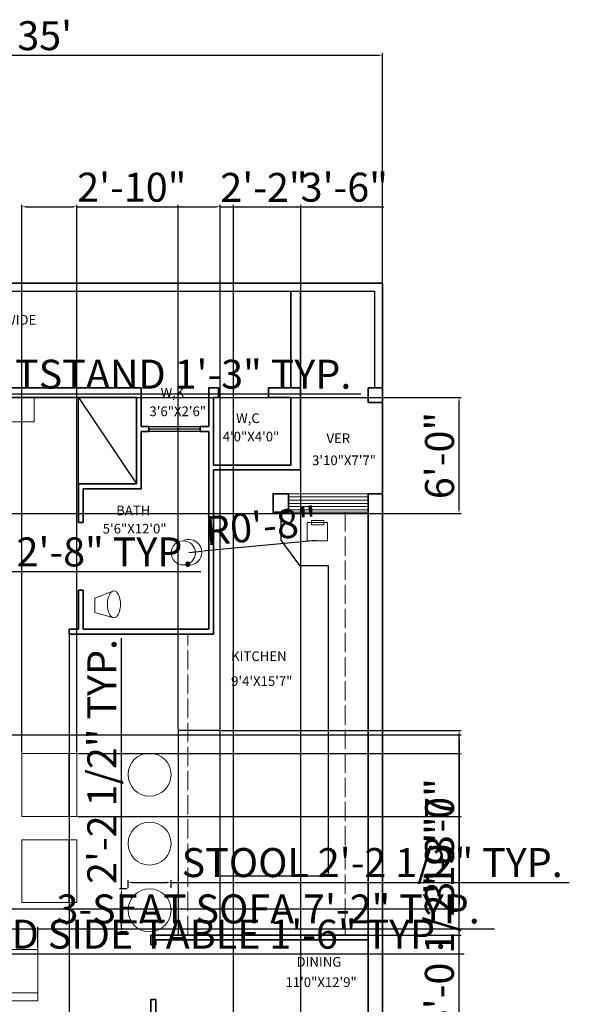
# Model space of a CAD drawing. Units: inches. Extents: x 2484 to 3244, y 1684 to 2692.
# Tile 3 of 3: x 2821 to 3162, y 2081 to 2692. Entities that reach past the tile are written whole.
import ezdxf

# ---------------------------------------------------------------- set-up
doc = ezdxf.new("R2010")
doc.units = ezdxf.units.IN
doc.linetypes.add('ACAD_ISO02W100', pattern=[15, 12, -3])
doc.layers.get('0').update_dxf_attribs({"color": 120})
for name, color, linetype, lineweight in [('A-ANNO-DIMS', 2, 'Continuous', 18), ('A-AREA-IDEN', 2, 'Continuous', 18), ('A-COLS', 120, 'Continuous', 35), ('A-FLOR-CASE', 120, 'Continuous', 25), ('A-FLOR-CASE-OVHD', 255, 'ACAD_ISO02W100', 18), ('A-FLOR-FIXT', 4, 'Continuous', 18), ('A-FURN', 40, 'Continuous', 18), ('A-GLAZ', 4, 'Continuous', 13), ('A-WALL', 120, 'Continuous', 35), ('A-WALL-OVHD', 255, 'ACAD_ISO02W100', 18), ('C-PROP', 120, 'Continuous', 35), ('C-SITE', 120, 'Continuous', 25)]:
    doc.layers.add(name, color=color, linetype=linetype, lineweight=lineweight)
doc.styles.get("Standard").update_dxf_attribs({"font": 'arial.ttf'})
doc.dimstyles.new('ISO-25', dxfattribs={"dimtxt": 18, "dimasz": 2.5, "dimexe": 1.25, "dimexo": 0.625, "dimtad": 1, "dimdec": 0, "dimlunit": 3, "dimtxsty": 'Standard', "dimcen": 2.5, "dimadec": 0, "dimazin": 0, "dimtfac": 1, "dimtdec": 0, "dimtmove": 0, "dimatfit": 3, "dimfxl": 1, "dimarcsym": 0})

# ---------------------------------------------------------------- blocks, each defined once
blk = doc.blocks.new('*D1')
at = {"layer": 'A-ANNO-DIMS', "color": 0, "lineweight": -2, "transparency": 16777216}
for p, q in [((2626.09, 2529.34), (2626.09, 2671.64)), ((2628.59, 2670.39), (3043.59, 2670.39)), ((3046.09, 2529.34), (3046.09, 2671.64))]:
    blk.add_line(p, q, dxfattribs=at)
at = {"layer": 'A-ANNO-DIMS', "color": 0, "transparency": 16777216}
for points in [[(2628.59, 2670.81), (2628.59, 2669.97), (2626.09, 2670.39)], [(3043.59, 2670.81), (3043.59, 2669.97), (3046.09, 2670.39)]]:
    blk.add_solid(points, dxfattribs=at)
at = {"layer": 'Defpoints', "color": 0, "transparency": 16777216}
for p in [(3046.09, 2670.39), (2626.09, 2528.71), (3046.09, 2528.71)]:
    blk.add_point(p, dxfattribs=at)
at = {"layer": 'A-ANNO-DIMS', "color": 0, "transparency": 16777216, "insert": (2836.09, 2680.21), "char_height": 18, "attachment_point": 5}
blk.add_mtext("35'", dxfattribs=at)
blk = doc.blocks.new('SOFA-3')
for p, q in [((0.07, 0), (0.07, 32)), ((0.07, 32), (86.07, 32)), ((29.07, 0), (29.07, 32)), ((58.07, 0), (58.07, 32)), ((86.07, 32), (86.07, 0)), ((0.07, 0), (0, 5)), ((0, 5), (86.07, 5)), ((0.07, 0), (0.07, 5)), ((86.07, 0), (0.07, 0))]:
    blk.add_line(p, q)
blk = doc.blocks.new('STOOL')
blk.add_circle((0, 0), 13.36)
blk = doc.blocks.new('NIGHTSTAND-15')
blk.add_lwpolyline([(15, 15), (0, 15), (0, 0), (15, 0)], close=True)
blk = doc.blocks.new('*D9')
at = {"layer": 'A-ANNO-DIMS', "color": 0, "lineweight": -2, "transparency": 16777216}
for p, q in [((2714.44, 2109.91), (2714.44, 2113.27)), ((2716.94, 2112.02), (2730.14, 2112.02)), ((2732.64, 2109.91), (2732.64, 2113.27)), ((2732.64, 2112.02), (3096.69, 2112.02))]:
    blk.add_line(p, q, dxfattribs=at)
at = {"layer": 'A-ANNO-DIMS', "color": 0, "transparency": 16777216}
for points in [[(2716.94, 2112.44), (2716.94, 2111.6), (2714.44, 2112.02)], [(2730.14, 2112.44), (2730.14, 2111.6), (2732.64, 2112.02)]]:
    blk.add_solid(points, dxfattribs=at)
at = {"layer": 'Defpoints', "color": 0, "transparency": 16777216}
for p in [(2732.64, 2112.02), (2714.44, 2109.29), (2732.64, 2109.29)]:
    blk.add_point(p, dxfattribs=at)
at = {"layer": 'A-ANNO-DIMS', "color": 0, "transparency": 16777216, "insert": (2915.92, 2121.96), "char_height": 18, "attachment_point": 5}
blk.add_mtext('ROUND SIDE TABLE 1\'-6" TYP.', dxfattribs=at)
blk = doc.blocks.new('*D11')
at = {"layer": 'A-ANNO-DIMS', "color": 0, "lineweight": -2, "transparency": 16777216}
for p, q in [((2887.88, 2153.12), (2887.88, 2157.76)), ((2890.38, 2156.51), (2912.09, 2156.51)), ((2914.59, 2153.12), (2914.59, 2157.76)), ((2914.59, 2156.51), (3162.14, 2156.51))]:
    blk.add_line(p, q, dxfattribs=at)
at = {"layer": 'A-ANNO-DIMS', "color": 0, "transparency": 16777216}
for points in [[(2890.38, 2156.92), (2890.38, 2156.09), (2887.88, 2156.51)], [(2912.09, 2156.92), (2912.09, 2156.09), (2914.59, 2156.51)]]:
    blk.add_solid(points, dxfattribs=at)
at = {"layer": 'Defpoints', "color": 0, "transparency": 16777216}
for p in [(2914.59, 2156.51), (2887.88, 2152.5), (2914.59, 2152.5)]:
    blk.add_point(p, dxfattribs=at)
at = {"layer": 'A-ANNO-DIMS', "color": 0, "transparency": 16777216, "insert": (3039.62, 2166.45), "char_height": 18, "attachment_point": 5}
blk.add_mtext('STOOL 2\'-2 1/2" TYP.', dxfattribs=at)
blk = doc.blocks.new('*D12')
at = {"layer": 'A-ANNO-DIMS', "color": 0, "lineweight": -2, "transparency": 16777216}
for p, q in [((2883.87, 2152.5), (2883.87, 2308.22)), ((2887.25, 2152.5), (2882.62, 2152.5)), ((2883.87, 2128.28), (2883.87, 2150)), ((2887.25, 2125.78), (2882.62, 2125.78))]:
    blk.add_line(p, q, dxfattribs=at)
at = {"layer": 'A-ANNO-DIMS', "color": 0, "transparency": 16777216}
for points in [[(2883.45, 2150), (2884.29, 2150), (2883.87, 2152.5)], [(2883.45, 2128.28), (2884.29, 2128.28), (2883.87, 2125.78)]]:
    blk.add_solid(points, dxfattribs=at)
at = {"layer": 'Defpoints', "color": 0, "transparency": 16777216}
for p in [(2883.87, 2152.5), (2887.88, 2152.5), (2887.88, 2125.78)]:
    blk.add_point(p, dxfattribs=at)
at = {"layer": 'A-ANNO-DIMS', "color": 0, "transparency": 16777216, "insert": (2873.94, 2231.61), "char_height": 18, "attachment_point": 5, "rotation": 90}
blk.add_mtext('2\'-2 1/2" TYP.', dxfattribs=at)
blk = doc.blocks.new('*D13')
at = {"layer": 'A-ANNO-DIMS', "color": 0, "lineweight": -2, "transparency": 16777216}
for p, q in [((2745.68, 2115.42), (2745.68, 2128.95)), ((2831.75, 2115.42), (2831.75, 2128.95)), ((2748.18, 2127.7), (2829.25, 2127.7)), ((2831.75, 2127.7), (3115.68, 2127.7))]:
    blk.add_line(p, q, dxfattribs=at)
at = {"layer": 'A-ANNO-DIMS', "color": 0, "transparency": 16777216}
for points in [[(2748.18, 2128.12), (2748.18, 2127.28), (2745.68, 2127.7)], [(2829.25, 2128.12), (2829.25, 2127.28), (2831.75, 2127.7)]]:
    blk.add_solid(points, dxfattribs=at)
at = {"layer": 'Defpoints', "color": 0, "transparency": 16777216}
for p in [(2831.75, 2127.7), (2745.68, 2114.79), (2831.75, 2114.79)]:
    blk.add_point(p, dxfattribs=at)
at = {"layer": 'A-ANNO-DIMS', "color": 0, "transparency": 16777216, "insert": (2974.96, 2137.65), "char_height": 18, "attachment_point": 5}
blk.add_mtext('3-SEAT SOFA 7\'-2" TYP.', dxfattribs=at)
blk = doc.blocks.new('*D17')
at = {"layer": 'A-ANNO-DIMS', "color": 0, "lineweight": -2, "transparency": 16777216}
for p, q in [((2702.65, 2345.36), (2702.65, 2350.79)), ((2705.15, 2349.54), (2732.15, 2349.54)), ((2734.65, 2345.36), (2734.65, 2350.79)), ((2734.65, 2349.54), (2933.13, 2349.54))]:
    blk.add_line(p, q, dxfattribs=at)
at = {"layer": 'A-ANNO-DIMS', "color": 0, "transparency": 16777216}
for points in [[(2705.15, 2349.96), (2705.15, 2349.12), (2702.65, 2349.54)], [(2732.15, 2349.96), (2732.15, 2349.12), (2734.65, 2349.54)]]:
    blk.add_solid(points, dxfattribs=at)
at = {"layer": 'Defpoints', "color": 0, "transparency": 16777216}
for p in [(2734.65, 2349.54), (2702.65, 2344.74), (2734.65, 2344.74)]:
    blk.add_point(p, dxfattribs=at)
at = {"layer": 'A-ANNO-DIMS', "color": 0, "transparency": 16777216, "insert": (2835.14, 2359.47), "char_height": 18, "attachment_point": 5}
blk.add_mtext('CHAIR 2\'-8" TYP.', dxfattribs=at)
blk = doc.blocks.new('*D19')
at = {"layer": 'A-ANNO-DIMS', "color": 0, "lineweight": -2, "transparency": 16777216}
for p, q in [((2734.51, 2458.34), (2734.51, 2461.21)), ((2737.01, 2459.96), (2747.01, 2459.96)), ((2749.51, 2458.34), (2749.51, 2461.21)), ((2749.51, 2459.96), (3032.54, 2459.96))]:
    blk.add_line(p, q, dxfattribs=at)
at = {"layer": 'A-ANNO-DIMS', "color": 0, "transparency": 16777216}
for points in [[(2737.01, 2460.38), (2737.01, 2459.55), (2734.51, 2459.96)], [(2747.01, 2460.38), (2747.01, 2459.55), (2749.51, 2459.96)]]:
    blk.add_solid(points, dxfattribs=at)
at = {"layer": 'Defpoints', "color": 0, "transparency": 16777216}
for p in [(2749.51, 2459.96), (2734.51, 2457.71), (2749.51, 2457.71)]:
    blk.add_point(p, dxfattribs=at)
at = {"layer": 'A-ANNO-DIMS', "color": 0, "transparency": 16777216, "insert": (2892.27, 2469.9), "char_height": 18, "attachment_point": 5}
blk.add_mtext('NIGHTSTAND 1\'-3" TYP.', dxfattribs=at)
blk = doc.blocks.new('*D22')
at = {"layer": 'A-ANNO-DIMS', "color": 0, "lineweight": -2, "transparency": 16777216}
for p, q in [((2815.13, 2457.71), (3094.89, 2457.71)), ((3093.64, 2388.21), (3093.64, 2455.21)), ((2815.13, 2385.71), (3094.89, 2385.71))]:
    blk.add_line(p, q, dxfattribs=at)
at = {"layer": 'A-ANNO-DIMS', "color": 0, "transparency": 16777216}
for points in [[(3093.22, 2455.21), (3094.05, 2455.21), (3093.64, 2457.71)], [(3093.22, 2388.21), (3094.05, 2388.21), (3093.64, 2385.71)]]:
    blk.add_solid(points, dxfattribs=at)
at = {"layer": 'Defpoints', "color": 0, "transparency": 16777216}
for p in [(2814.51, 2457.71), (3093.64, 2457.71), (2814.51, 2385.71)]:
    blk.add_point(p, dxfattribs=at)
at = {"layer": 'A-ANNO-DIMS', "color": 0, "transparency": 16777216, "insert": (3083.82, 2421.71), "char_height": 18, "attachment_point": 5, "rotation": 90}
blk.add_mtext('6\'-0"', dxfattribs=at)
blk = doc.blocks.new('*D23')
at = {"layer": 'A-ANNO-DIMS', "color": 0, "lineweight": -2, "transparency": 16777216}
for p, q in [((2953.42, 2064.92), (2953.42, 2577.51)), ((2955.92, 2576.26), (2992.74, 2576.26)), ((2995.24, 2064.92), (2995.24, 2577.51)), ((2995.24, 2576.26), (3046.83, 2576.26))]:
    blk.add_line(p, q, dxfattribs=at)
at = {"layer": 'A-ANNO-DIMS', "color": 0, "transparency": 16777216}
for points in [[(2955.92, 2576.68), (2955.92, 2575.85), (2953.42, 2576.26)], [(2992.74, 2576.68), (2992.74, 2575.85), (2995.24, 2576.26)]]:
    blk.add_solid(points, dxfattribs=at)
at = {"layer": 'Defpoints', "color": 0, "transparency": 16777216}
for p in [(2995.24, 2576.26), (2953.42, 2064.3), (2995.24, 2064.3)]:
    blk.add_point(p, dxfattribs=at)
at = {"layer": 'A-ANNO-DIMS', "color": 0, "transparency": 16777216, "insert": (3022.28, 2586.08), "char_height": 18, "attachment_point": 5}
blk.add_mtext('3\'-6"', dxfattribs=at)
blk = doc.blocks.new('*D24')
at = {"layer": 'A-ANNO-DIMS', "color": 0, "lineweight": -2, "transparency": 16777216}
for p, q in [((3093.64, 2064.3), (3093.64, 2157.84)), ((2995.86, 2064.3), (3094.89, 2064.3)), ((3093.64, 2006.27), (3093.64, 2061.8)), ((2995.86, 2003.77), (3094.89, 2003.77))]:
    blk.add_line(p, q, dxfattribs=at)
at = {"layer": 'A-ANNO-DIMS', "color": 0, "transparency": 16777216}
for points in [[(3093.22, 2061.8), (3094.05, 2061.8), (3093.64, 2064.3)], [(3093.22, 2006.27), (3094.05, 2006.27), (3093.64, 2003.77)]]:
    blk.add_solid(points, dxfattribs=at)
at = {"layer": 'Defpoints', "color": 0, "transparency": 16777216}
for p in [(2995.24, 2064.3), (3093.64, 2064.3), (2995.24, 2003.77)]:
    blk.add_point(p, dxfattribs=at)
at = {"layer": 'A-ANNO-DIMS', "color": 0, "transparency": 16777216, "insert": (3083.71, 2112.32), "char_height": 18, "attachment_point": 5, "rotation": 90}
blk.add_mtext('5\'-0 1/2"', dxfattribs=at)
blk = doc.blocks.new('*D31')
at = {"layer": 'A-ANNO-DIMS', "color": 0, "lineweight": -2, "transparency": 16777216}
for p, q in [((2705.68, 2248.09), (3094.89, 2248.09)), ((3093.64, 2245.59), (3093.64, 2142.59)), ((2705.68, 2140.09), (3094.89, 2140.09))]:
    blk.add_line(p, q, dxfattribs=at)
at = {"layer": 'A-ANNO-DIMS', "color": 0, "transparency": 16777216}
for points in [[(3093.22, 2245.59), (3094.05, 2245.59), (3093.64, 2248.09)], [(3093.22, 2142.59), (3094.05, 2142.59), (3093.64, 2140.09)]]:
    blk.add_solid(points, dxfattribs=at)
at = {"layer": 'Defpoints', "color": 0, "transparency": 16777216}
for p in [(2705.05, 2248.09), (2705.05, 2140.09), (3093.64, 2140.09)]:
    blk.add_point(p, dxfattribs=at)
at = {"layer": 'A-ANNO-DIMS', "color": 0, "transparency": 16777216, "insert": (3083.82, 2194.09), "char_height": 18, "attachment_point": 5, "rotation": 90}
blk.add_mtext('9\'-0"', dxfattribs=at)
blk = doc.blocks.new('*D33')
at = {"layer": 'A-ANNO-DIMS', "color": 0, "lineweight": -2, "transparency": 16777216}
for p, q in [((2821.96, 2237.17), (2821.96, 2577.51)), ((2824.46, 2576.26), (2853.53, 2576.26)), ((2856.03, 2237.17), (2856.03, 2577.51)), ((2856.03, 2576.26), (2921.92, 2576.26))]:
    blk.add_line(p, q, dxfattribs=at)
at = {"layer": 'A-ANNO-DIMS', "color": 0, "transparency": 16777216}
for points in [[(2824.46, 2576.68), (2824.46, 2575.85), (2821.96, 2576.26)], [(2853.53, 2576.68), (2853.53, 2575.85), (2856.03, 2576.26)]]:
    blk.add_solid(points, dxfattribs=at)
at = {"layer": 'Defpoints', "color": 0, "transparency": 16777216}
for p in [(2856.03, 2576.26), (2821.96, 2236.54), (2856.03, 2236.54)]:
    blk.add_point(p, dxfattribs=at)
at = {"layer": 'A-ANNO-DIMS', "color": 0, "transparency": 16777216, "insert": (2890.23, 2586.08), "char_height": 18, "attachment_point": 5}
blk.add_mtext('2\'-10"', dxfattribs=at)
blk = doc.blocks.new('*D34')
at = {"layer": 'A-ANNO-DIMS', "color": 0, "lineweight": -2, "transparency": 16777216}
for p, q in [((2856.66, 2236.54), (3094.89, 2236.54)), ((3093.64, 2234.04), (3093.64, 2199.97)), ((2856.66, 2197.47), (3094.89, 2197.47)), ((3093.64, 2197.47), (3093.64, 2145.88))]:
    blk.add_line(p, q, dxfattribs=at)
at = {"layer": 'A-ANNO-DIMS', "color": 0, "transparency": 16777216}
for points in [[(3093.22, 2234.04), (3094.05, 2234.04), (3093.64, 2236.54)], [(3093.22, 2199.97), (3094.05, 2199.97), (3093.64, 2197.47)]]:
    blk.add_solid(points, dxfattribs=at)
at = {"layer": 'Defpoints', "color": 0, "transparency": 16777216}
for p in [(2856.03, 2236.54), (2856.03, 2197.47), (3093.64, 2197.47)]:
    blk.add_point(p, dxfattribs=at)
at = {"layer": 'A-ANNO-DIMS', "color": 0, "transparency": 16777216, "insert": (3083.82, 2170.43), "char_height": 18, "attachment_point": 5, "rotation": 90}
blk.add_mtext('3\'-3"', dxfattribs=at)
blk = doc.blocks.new('*D37')
at = {"layer": 'A-ANNO-DIMS', "color": 0, "lineweight": -2, "transparency": 16777216}
for p, q in [((2799.42, 2313.09), (2799.42, 1699.91)), ((2851.28, 2313.09), (2851.28, 1699.91)), ((2801.92, 1701.16), (2848.78, 1701.16))]:
    blk.add_line(p, q, dxfattribs=at)
at = {"layer": 'A-ANNO-DIMS', "color": 0, "transparency": 16777216}
for points in [[(2801.92, 1701.58), (2801.92, 1700.75), (2799.42, 1701.16)], [(2848.78, 1701.58), (2848.78, 1700.75), (2851.28, 1701.16)]]:
    blk.add_solid(points, dxfattribs=at)
at = {"layer": 'Defpoints', "color": 0, "transparency": 16777216}
for p in [(2799.42, 2313.71), (2851.28, 2313.71), (2851.28, 1701.16)]:
    blk.add_point(p, dxfattribs=at)
at = {"layer": 'A-ANNO-DIMS', "color": 0, "transparency": 16777216, "insert": (2825.35, 1710.79), "char_height": 18, "attachment_point": 5}
blk.add_mtext('4\'-4"', dxfattribs=at)
blk = doc.blocks.new('*D39')
at = {"layer": 'A-ANNO-DIMS', "color": 0, "lineweight": -2, "transparency": 16777216}
for p, q in [((2919.09, 2251.56), (2919.09, 2577.51)), ((2921.59, 2576.26), (2942.66, 2576.26)), ((2945.16, 2251.56), (2945.16, 2577.51)), ((2945.16, 2576.26), (2997.07, 2576.26))]:
    blk.add_line(p, q, dxfattribs=at)
at = {"layer": 'A-ANNO-DIMS', "color": 0, "transparency": 16777216}
for points in [[(2921.59, 2576.68), (2921.59, 2575.85), (2919.09, 2576.26)], [(2942.66, 2576.68), (2942.66, 2575.85), (2945.16, 2576.26)]]:
    blk.add_solid(points, dxfattribs=at)
at = {"layer": 'Defpoints', "color": 0, "transparency": 16777216}
for p in [(2945.16, 2576.26), (2919.09, 2250.94), (2945.16, 2250.94)]:
    blk.add_point(p, dxfattribs=at)
at = {"layer": 'A-ANNO-DIMS', "color": 0, "transparency": 16777216, "insert": (2972.36, 2585.93), "char_height": 18, "attachment_point": 5}
blk.add_mtext('2\'-2"', dxfattribs=at)
blk = doc.blocks.new('*D40')
at = {"layer": 'A-ANNO-DIMS', "color": 0, "lineweight": -2, "transparency": 16777216}
for p, q in [((2945.79, 2250.94), (3094.89, 2250.94)), ((3093.64, 2126.21), (3093.64, 2248.44)), ((2945.79, 2123.71), (3094.89, 2123.71))]:
    blk.add_line(p, q, dxfattribs=at)
at = {"layer": 'A-ANNO-DIMS', "color": 0, "transparency": 16777216}
for points in [[(3093.22, 2248.44), (3094.05, 2248.44), (3093.64, 2250.94)], [(3093.22, 2126.21), (3094.05, 2126.21), (3093.64, 2123.71)]]:
    blk.add_solid(points, dxfattribs=at)
at = {"layer": 'Defpoints', "color": 0, "transparency": 16777216}
for p in [(2945.16, 2250.94), (3093.64, 2250.94), (2945.16, 2123.71)]:
    blk.add_point(p, dxfattribs=at)
at = {"layer": 'A-ANNO-DIMS', "color": 0, "transparency": 16777216, "insert": (3083.82, 2187.33), "char_height": 18, "attachment_point": 5, "rotation": 90}
blk.add_mtext('10\'-7"', dxfattribs=at)
blk = doc.blocks.new('*D41')
at = {"layer": 'A-ANNO-DIMS', "color": 0, "lineweight": -2, "transparency": 16777216}
for p, q in [((3004.71, 2368.85), (2936.18, 2362.5)), ((2925.73, 2361.54), (2933.69, 2362.27))]:
    blk.add_line(p, q, dxfattribs=at)
at = {"layer": 'A-ANNO-DIMS', "color": 0, "transparency": 16777216}
blk.add_solid([(2936.14, 2362.92), (2936.22, 2362.09), (2933.69, 2362.27)], dxfattribs=at)
at = {"layer": 'Defpoints', "color": 0, "transparency": 16777216}
for p in [(2925.73, 2361.54), (2933.69, 2362.27)]:
    blk.add_point(p, dxfattribs=at)
at = {"layer": 'A-ANNO-DIMS', "color": 0, "transparency": 16777216, "insert": (2970.79, 2375.57), "char_height": 18, "attachment_point": 5, "rotation": 5.28891}
blk.add_mtext('R0\'-8"', dxfattribs=at)

msp = doc.modelspace()

# ---------------------------------------------------------------- linework, layer by layer
at = {"layer": 'A-COLS'}
msp.add_lwpolyline([(2987.58, 2397.94), (2977.99, 2397.94), (2977.99, 2386.45), (2987.58, 2386.45)], close=True, dxfattribs=at)
at = {"layer": 'A-FLOR-CASE'}
for p, q in [((2857.09, 2404.08), (2857.09, 2457.71)), ((2857.09, 2457.71), (2893.09, 2404.08)), ((2982.78, 2386.45), (2982.78, 2369.09)), ((2982.78, 2369.09), (2994.39, 2353.45)), ((2994.39, 2353.45), (3012.33, 2353.45)), ((3012.33, 2353.45), (3012.33, 2160.37)), ((3012.33, 2160.37), (2945.16, 2160.37))]:
    msp.add_line(p, q, dxfattribs=at)
msp.add_lwpolyline([(2919.09, 2123.71), (2945.16, 2123.71), (2945.16, 2250.94), (2919.09, 2250.94)], close=True, dxfattribs=at)
at = {"layer": 'A-FLOR-CASE-OVHD'}
msp.add_line((3022.92, 2386.45), (3022.92, 2123.71), dxfattribs=at)
at = {"layer": 'A-FLOR-FIXT'}
for p, q in [((2879.13, 2337.66), (2867.27, 2333.03)), ((2867.27, 2333.03), (2867.27, 2324.07)), ((2867.27, 2324.07), (2879.13, 2320.89))]:
    msp.add_line(p, q, dxfattribs=at)
for points in [[(2999.24, 2380.02), (3011.92, 2380.02), (3011.92, 2368.62), (2999.24, 2368.62)], [(3001.93, 2381.25), (3009.65, 2381.25), (3009.65, 2378.63), (3001.93, 2378.63)]]:
    msp.add_lwpolyline(points, close=True, dxfattribs=at)
msp.add_circle((2922.22, 2361.21), 7.51, dxfattribs=at)
msp.add_arc((2925.73, 2361.54), 8, 254.60149, 115.98031, dxfattribs=at)
msp.add_ellipse((2879.13, 2329.28), major_axis=(0, -8.39), ratio=0.482758, dxfattribs=at)
at = {"layer": 'A-FURN'}
for p, q in [((2856.03, 2236.54), (2851.04, 2236.26)), ((2851.04, 2236.26), (2851.04, 2197.47)), ((2851.04, 2182.97), (2851.04, 2143.89))]:
    msp.add_line(p, q, dxfattribs=at)
for points in [[(2821.96, 2197.47), (2856.03, 2197.47), (2856.03, 2236.54), (2821.96, 2236.54)], [(2821.96, 2143.89), (2856.03, 2143.89), (2856.03, 2182.97), (2821.96, 2182.97)]]:
    msp.add_lwpolyline(points, close=True, dxfattribs=at)
at = {"layer": 'A-GLAZ'}
for p, q in [((2900.73, 2439.71), (2932.65, 2439.71)), ((2900.73, 2438.71), (2932.65, 2438.71)), ((2900.73, 2437.71), (2932.65, 2437.71)), ((2900.73, 2436.71), (2932.65, 2436.71)), ((2987.58, 2397.94), (3037.09, 2397.94)), ((2987.58, 2395.94), (3037.09, 2395.94)), ((2987.58, 2393.94), (3037.09, 2393.94)), ((2987.58, 2391.94), (3037.09, 2391.94)), ((2987.58, 2389.94), (3037.09, 2389.94)), ((2987.58, 2387.94), (3037.09, 2387.94)), ((2987.58, 2386.45), (3037.09, 2386.45))]:
    msp.add_line(p, q, dxfattribs=at)
at = {"layer": 'A-WALL'}
for p, q in [((2989.09, 2523.71), (2989.09, 2463.71)), ((2995.09, 2523.71), (2995.09, 2412.71)), ((2691.09, 2463.71), (2896.09, 2463.71)), ((2896.09, 2463.71), (2896.09, 2439.71)), ((2938.09, 2463.71), (2938.09, 2439.71)), ((2938.09, 2463.71), (2944.09, 2463.71)), ((2944.09, 2463.71), (2944.09, 2457.71)), ((2975.09, 2463.71), (2995.09, 2463.71)), ((2975.09, 2457.71), (2975.09, 2463.71)), ((3037.09, 2463.71), (3037.09, 2454.71)), ((3037.09, 2463.71), (3037.09, 2454.71)), ((3037.09, 2463.71), (3041.09, 2463.71)), ((3046.09, 2463.71), (3041.09, 2463.71)), ((3046.09, 2454.71), (3046.09, 2463.71)), ((2697.09, 2457.71), (2893.09, 2457.71)), ((2893.09, 2457.71), (2893.09, 2404.08)), ((2941.09, 2457.71), (2941.09, 2415.71)), ((2941.09, 2457.71), (2944.09, 2457.71)), ((2975.09, 2457.71), (2989.09, 2457.71)), ((2989.09, 2457.71), (2989.09, 2415.71)), ((3037.09, 2454.71), (3046.09, 2454.71)), ((2900.73, 2439.71), (2896.09, 2439.71)), ((2900.73, 2436.71), (2896.09, 2436.71)), ((2896.09, 2436.71), (2896.09, 2401.08)), ((2900.73, 2439.71), (2900.73, 2436.71)), ((2938.09, 2439.71), (2932.65, 2439.71)), ((2932.65, 2439.71), (2932.65, 2436.71)), ((2938.09, 2436.71), (2932.65, 2436.71)), ((2938.09, 2436.71), (2938.09, 2313.71)), ((2941.09, 2415.71), (2989.09, 2415.71)), ((2941.09, 2412.71), (2995.09, 2412.71)), ((2941.09, 2412.71), (2941.09, 2310.71)), ((2893.09, 2404.08), (2857.09, 2404.08)), ((2857.09, 2404.08), (2857.09, 2380.08)), ((2857.09, 2401.08), (2857.09, 2380.08)), ((2860.09, 2380.08), (2860.09, 2401.08)), ((2860.09, 2401.08), (2896.09, 2401.08)), ((2860.09, 2401.08), (2860.09, 2380.08)), ((3037.09, 2397.94), (3046.09, 2397.94)), ((3037.09, 2397.94), (3037.09, 1973.56)), ((2857.09, 2380.08), (2860.09, 2380.08)), ((2857.09, 2338.08), (2860.09, 2338.08)), ((2857.09, 2338.08), (2857.09, 2313.71)), ((2860.09, 2338.08), (2860.09, 2313.71)), ((2851.28, 2313.71), (2851.28, 2310.71)), ((2851.28, 2313.71), (2857.09, 2313.71)), ((2860.09, 2313.71), (2938.09, 2313.71)), ((2851.28, 2310.71), (2941.09, 2310.71)), ((2902.09, 2123.71), (3037.09, 2123.71)), ((2902.09, 2123.71), (2902.09, 2117.71)), ((2905.09, 2117.71), (2902.09, 2117.71)), ((2905.09, 2120.71), (3037.09, 2120.71)), ((2905.09, 2120.71), (2905.09, 2117.71)), ((2905.09, 2120.71), (2905.09, 2117.71)), ((2905.09, 2083.7), (2902.09, 2083.7)), ((2902.09, 2083.7), (2902.09, 2071.85)), ((2905.09, 2083.7), (2905.09, 2065.85))]:
    msp.add_line(p, q, dxfattribs=at)
at = {"layer": 'A-WALL-OVHD'}
for p, q in [((2919.09, 2310.71), (2919.09, 2123.71)), ((2925.09, 2123.71), (2925.09, 2310.71))]:
    msp.add_line(p, q, dxfattribs=at)
at = {"layer": 'C-PROP'}
msp.add_lwpolyline([(2626.09, 2528.71), (3046.09, 2528.71), (3046.09, 1748.71), (2626.09, 1748.71)], close=True, dxfattribs=at)
at = {"layer": 'C-SITE'}
for p, q in [((2631.09, 2523.71), (3041.09, 2523.71)), ((3041.09, 2523.71), (3041.09, 2463.71))]:
    msp.add_line(p, q, dxfattribs=at)

# ---------------------------------------------------------------- block references
at = {"layer": 'A-FURN'}
for name, p in [('NIGHTSTAND-15', (2814.51, 2442.71)), ('STOOL', (2901.24, 2223.44)), ('STOOL', (2901.24, 2180.6)), ('STOOL', (2901.24, 2139.14)), ('SOFA-3', (2745.68, 2082.79))]:
    msp.add_blockref(name, p, dxfattribs=at)

# ---------------------------------------------------------------- texts
at = {"layer": 'A-AREA-IDEN'}
for tag, p in [('5\'-4"WIDE', (2792.76, 2503.01)), ('W,K', (2908.14, 2457.7)), ('3\'6"X2\'6"', (2901.2, 2446.14)), ('W,C', (2955.05, 2441.88)), ('4\'0"X4\'0"', (2946.72, 2430.48)), ('VER', (3011.23, 2429.4)), ('3\'10"X7\'7"', (3002.28, 2415.71)), ('BATH', (2880.51, 2384.57)), ('5\'6"X12\'0"', (2872.13, 2373.25)), ('KITCHEN', (2951.94, 2294)), ('9\'4\'X15\'7"', (2951.94, 2278.53)), ('DINING', (2992.59, 2104.11)), ('11\'0"X12\'9"', (2985.76, 2091.49))]:
    msp.add_attdef(tag, p, '', height=6, dxfattribs=at)

# ---------------------------------------------------------------- dimensions: what is measured, and where the dimension line sits
at = {"layer": 'A-ANNO-DIMS'}
for base, p1, p2, override, picture, middle in [((3046.09, 2670.39), (2626.09, 2528.71), (3046.09, 2528.71), {"dimclrd": 0, "dimclre": 0, "dimclrt": 0}, '*D1', (2836.09, 2680.21)), ((2856.03, 2576.26), (2821.96, 2236.54), (2856.03, 2236.54), {"dimdec": 1, "dimlfac": 1, "dimrnd": 0, "dimzin": 1, "dimdsep": 46, "dimlunit": 4, "dimfrac": 2}, '*D33', (2890.23, 2586.08)), ((2945.16, 2576.26), (2919.09, 2250.94), (2945.16, 2250.94), {"dimdec": 1, "dimlfac": 1, "dimrnd": 0, "dimzin": 1, "dimdsep": 46, "dimlunit": 4, "dimfrac": 2}, '*D39', (2972.36, 2585.93)), ((2995.24, 2576.26), (2953.42, 2064.3), (2995.24, 2064.3), {"dimdec": 1, "dimlfac": 1, "dimrnd": 0, "dimzin": 1, "dimdsep": 46, "dimlunit": 4, "dimfrac": 2}, '*D23', (3022.28, 2586.08)), ((2851.28, 1701.16), (2799.42, 2313.71), (2851.28, 2313.71), {"dimdec": 1, "dimlfac": 1, "dimrnd": 0, "dimzin": 1, "dimdsep": 46, "dimlunit": 4, "dimfrac": 2}, '*D37', (2825.35, 1710.79))]:
    dim = msp.add_linear_dim(base=base, p1=p1, p2=p2, dimstyle='ISO-25', override=override, dxfattribs=at)
    dim.commit()
    dim.dimension.update_dxf_attribs({"geometry": picture, "text_midpoint": middle})
for base, p1, p2, text, picture, middle in [((2749.51, 2459.96), (2734.51, 2457.71), (2749.51, 2457.71), 'NIGHTSTAND <> TYP.', '*D19', (2892.27, 2469.9)), ((2734.65, 2349.54), (2702.65, 2344.74), (2734.65, 2344.74), 'CHAIR <> TYP.', '*D17', (2835.14, 2359.47)), ((2914.59, 2156.51), (2887.88, 2152.5), (2914.59, 2152.5), 'STOOL <> TYP.', '*D11', (3039.62, 2166.45)), ((2732.64, 2112.02), (2714.44, 2109.29), (2732.64, 2109.29), 'ROUND SIDE TABLE <> TYP.', '*D9', (2915.92, 2121.96)), ((2831.75, 2127.7), (2745.68, 2114.79), (2831.75, 2114.79), '3-SEAT SOFA <> TYP.', '*D13', (2974.96, 2137.65))]:
    dim = msp.add_linear_dim(base=base, p1=p1, p2=p2, text=text, dimstyle='ISO-25', override={"dimdec": 1, "dimlfac": 1, "dimrnd": 0, "dimzin": 1, "dimdsep": 46, "dimlunit": 4, "dimfrac": 2}, dxfattribs=at)
    dim.commit()
    dim.dimension.update_dxf_attribs({"geometry": picture, "text_midpoint": middle})
for base, p1, p2, picture, middle in [((3093.64, 2457.71), (2814.51, 2385.71), (2814.51, 2457.71), '*D22', (3083.82, 2421.71)), ((3093.64, 2140.09), (2705.05, 2248.09), (2705.05, 2140.09), '*D31', (3083.82, 2194.09)), ((3093.64, 2250.94), (2945.16, 2123.71), (2945.16, 2250.94), '*D40', (3083.82, 2187.33)), ((3093.64, 2197.47), (2856.03, 2236.54), (2856.03, 2197.47), '*D34', (3083.82, 2170.43)), ((3093.64, 2064.3), (2995.24, 2003.77), (2995.24, 2064.3), '*D24', (3083.71, 2112.32))]:
    dim = msp.add_linear_dim(base=base, p1=p1, p2=p2, angle=90, dimstyle='ISO-25', override={"dimdec": 1, "dimlfac": 1, "dimrnd": 0, "dimzin": 1, "dimdsep": 46, "dimlunit": 4, "dimfrac": 2}, dxfattribs=at)
    dim.commit()
    dim.dimension.update_dxf_attribs({"geometry": picture, "text_midpoint": middle})
dim = msp.add_radius_dim(center=(2925.73, 2361.54), mpoint=(2933.69, 2362.27), dimstyle='ISO-25', override={"dimdec": 1, "dimlfac": 1, "dimrnd": 0, "dimzin": 1, "dimdsep": 46, "dimlunit": 4, "dimfrac": 2}, dxfattribs=at)
dim.commit()
dim.dimension.update_dxf_attribs({"geometry": '*D41', "text_midpoint": (2970.79, 2375.57)})
dim = msp.add_linear_dim(base=(2883.87, 2152.5), p1=(2887.88, 2125.78), p2=(2887.88, 2152.5), angle=90, text='<> TYP.', dimstyle='ISO-25', override={"dimdec": 1, "dimlfac": 1, "dimrnd": 0, "dimzin": 1, "dimdsep": 46, "dimlunit": 4, "dimfrac": 2}, dxfattribs=at)
dim.commit()
dim.dimension.update_dxf_attribs({"geometry": '*D12', "text_midpoint": (2873.94, 2231.61)})

doc.saveas('drawing.dxf')
